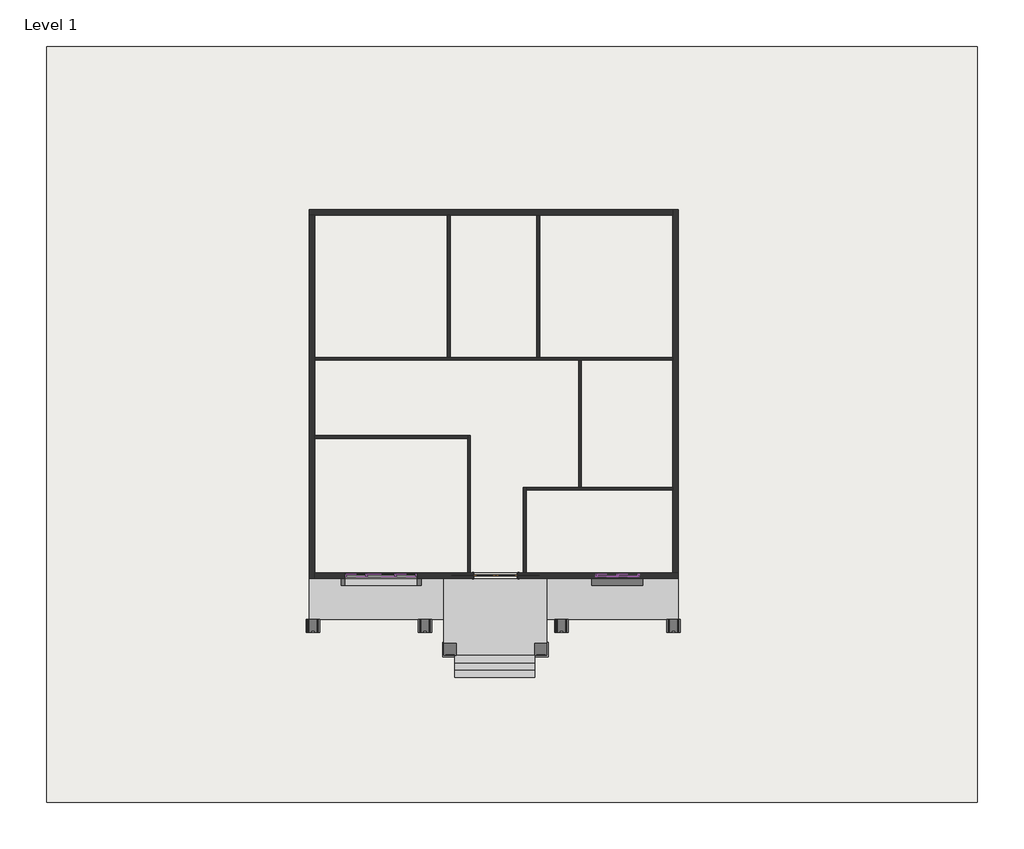
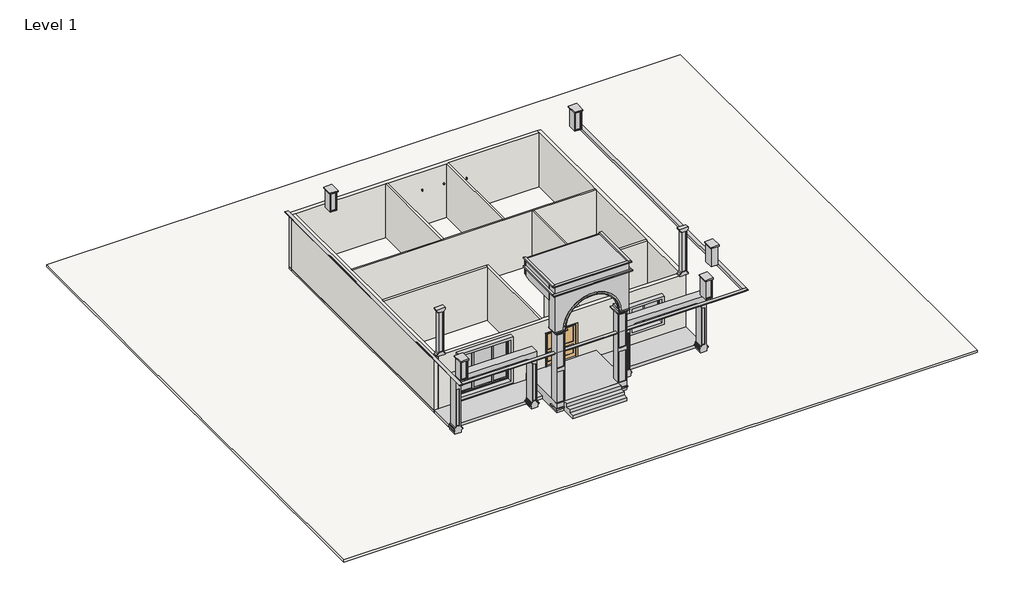
# One storey: 17 members, 12 walls, 5 plates, 2 slabs, 1 door, 1 proxy.
"""IFC4 building model written with IfcOpenShell, lengths in millimetres."""

from ifc_helpers import new_model, si_unit, frame, origin, origin_with_axes, place, context, project, spatial, polyline, outline, extrude, faceted_brep, transform, mapped, element, save
from components import generic_models_1_generic_models_1_83f40e1e, generic_models_1_generic_models_1_5e55def3, generic_models_1_generic_models_1_a6c1d6b2, door_c75fb906, member_c17f1be2, member_9661c287, member_d7472725, member_6ba65f20, member_82905deb, member_4491d118, system_panel_glazed_f88502f0, system_panel_glazed_214c7444, system_panel_glazed_e3982794

model = new_model("IFC4")

# Units and contexts
model_context = context("Model", 3, world=origin())
ifc_project = project(units=[si_unit("LENGTHUNIT", "METRE", prefix="MILLI")], contexts=[model_context])

# Site, building, storey
site = spatial("IfcSite", under=ifc_project)
building = spatial("IfcBuilding", under=site)
storey = spatial("IfcBuildingStorey", under=building, Name="Level 1", Elevation=0.0)

# Proxy
placement = place(None, origin())
generic_models_1_generic_models_1_shape = generic_models_1_generic_models_1_83f40e1e(model_context)
generic_models_1_generic_models_1_2_shape = generic_models_1_generic_models_1_5e55def3(model_context)
generic_models_1_generic_models_1_3_shape = generic_models_1_generic_models_1_a6c1d6b2(model_context)
element("IfcBuildingElementProxy", 1, Name="Generic Models 1 : Generic Models 1", ObjectType="Generic Models 1 : Generic Models 1", at=placement, inside=storey, context=model_context, shape_type="MappedRepresentation", body=[
    mapped(generic_models_1_generic_models_1_shape, transform((0.0, 0.0, 0.0), x_axis=(1.0, 0.0, 0.0), y_axis=(0.0, 1.0, 0.0), z_axis=(0.0, 0.0, 1.0))),
    mapped(generic_models_1_generic_models_1_2_shape, transform((0.0, 0.0, 0.0), x_axis=(1.0, 0.0, 0.0), y_axis=(0.0, 1.0, 0.0), z_axis=(0.0, 0.0, 1.0))),
    mapped(generic_models_1_generic_models_1_3_shape, transform((0.0, 0.0, 0.0), x_axis=(1.0, 0.0, 0.0), y_axis=(0.0, 1.0, 0.0), z_axis=(0.0, 0.0, 1.0))),
])

# Door
door_shape = door_c75fb906(model_context)
element("IfcDoor", 2, ObjectType="Door-Interior-Double-Pocket-2_Panel-Wood : 72\" x 84\"", at=placement, inside=storey, context=model_context, shape_type="MappedRepresentation", body=[
    mapped(door_shape, transform((-962.0249265, -5957.4949916, 609.6), x_axis=(-1.0, 0.0, 0.0), y_axis=(0.0, -1.0, 0.0), z_axis=(0.0, 0.0, 1.0))),
])

# Members
member_shape = member_c17f1be2(model_context)
element("IfcMember", 3, ObjectType="Rectangular Mullion : 2.5\" x 5\" rectangular", at=placement, inside=storey, context=model_context, shape_type="MappedRepresentation", body=[
    mapped(member_shape, transform((-4302.1249265, -5957.4949916, 3352.8), x_axis=(0.0, 0.0, 1.0), y_axis=(0.0, -1.0, 0.0), z_axis=(1.0, 0.0, 0.0))),
])
element("IfcMember", 4, ObjectType="Rectangular Mullion : 2.5\" x 5\" rectangular", at=placement, inside=storey, context=model_context, shape_type="MappedRepresentation", body=[
    mapped(member_shape, transform((-6403.9749265, -5957.4949916, 3352.8), x_axis=(0.0, 0.0, 1.0), y_axis=(0.0, -1.0, 0.0), z_axis=(1.0, 0.0, 0.0))),
])
element("IfcMember", 5, ObjectType="Rectangular Mullion : 2.5\" x 5\" rectangular", at=placement, inside=storey, context=model_context, shape_type="MappedRepresentation", body=[
    mapped(member_shape, transform((3292.4750735, -5957.4949916, 2743.2), x_axis=(0.0, 0.0, 1.0), y_axis=(0.0, 1.0, 0.0), z_axis=(-1.0, 0.0, 0.0))),
])
element("IfcMember", 6, ObjectType="Rectangular Mullion : 2.5\" x 5\" rectangular", at=placement, inside=storey, context=model_context, shape_type="MappedRepresentation", body=[
    mapped(member_shape, transform((4175.1250735, -5957.4949916, 2743.2), x_axis=(0.0, 0.0, 1.0), y_axis=(0.0, 1.0, 0.0), z_axis=(-1.0, 0.0, 0.0))),
])
element("IfcMember", 7, ObjectType="Rectangular Mullion : 2.5\" x 5\" rectangular", at=placement, inside=storey, context=model_context, shape_type="MappedRepresentation", body=[
    mapped(member_shape, transform((-7223.1249265, -5957.4949916, 685.8), x_axis=(0.0, 0.0, -1.0), y_axis=(0.0, -1.0, 0.0), z_axis=(-1.0, 0.0, 0.0))),
])
element("IfcMember", 8, ObjectType="Rectangular Mullion : 2.5\" x 5\" rectangular", at=placement, inside=storey, context=model_context, shape_type="MappedRepresentation", body=[
    mapped(member_shape, transform((-5121.2749265, -5957.4949916, 685.8), x_axis=(0.0, 0.0, -1.0), y_axis=(0.0, -1.0, 0.0), z_axis=(-1.0, 0.0, 0.0))),
])
element("IfcMember", 9, ObjectType="Rectangular Mullion : 2.5\" x 5\" rectangular", at=placement, inside=storey, context=model_context, shape_type="MappedRepresentation", body=[
    mapped(member_shape, transform((4994.2750735, -5957.4949916, 1219.2), x_axis=(0.0, 0.0, -1.0), y_axis=(0.0, 1.0, 0.0), z_axis=(1.0, 0.0, 0.0))),
])
element("IfcMember", 10, ObjectType="Rectangular Mullion : 2.5\" x 5\" rectangular", at=placement, inside=storey, context=model_context, shape_type="MappedRepresentation", body=[
    mapped(member_shape, transform((4111.6250735, -5957.4949916, 1219.2), x_axis=(0.0, 0.0, -1.0), y_axis=(0.0, 1.0, 0.0), z_axis=(1.0, 0.0, 0.0))),
])
member_2_shape = member_9661c287(model_context)
element("IfcMember", 11, ObjectType="Rectangular Mullion : 2.5\" x 5\" rectangular", at=placement, inside=storey, context=model_context, shape_type="MappedRepresentation", body=[
    mapped(member_2_shape, transform((-6372.2249265, -5957.4949916, 685.8), x_axis=(1.0, 0.0, 0.0), y_axis=(0.0, -1.0, 0.0), z_axis=(0.0, 0.0, -1.0))),
])
element("IfcMember", 12, ObjectType="Rectangular Mullion : 2.5\" x 5\" rectangular", at=placement, inside=storey, context=model_context, shape_type="MappedRepresentation", body=[
    mapped(member_2_shape, transform((-5153.0249265, -5957.4949916, 685.8), x_axis=(1.0, 0.0, 0.0), y_axis=(0.0, -1.0, 0.0), z_axis=(0.0, 0.0, -1.0))),
])
member_3_shape = member_d7472725(model_context)
element("IfcMember", 13, ObjectType="Rectangular Mullion : 2.5\" x 5\" rectangular", at=placement, inside=storey, context=model_context, shape_type="MappedRepresentation", body=[
    mapped(member_3_shape, transform((-6340.4749265, -5957.4949916, 685.8), x_axis=(0.0, 0.0, -1.0), y_axis=(0.0, -1.0, 0.0), z_axis=(-1.0, 0.0, 0.0))),
])
element("IfcMember", 14, ObjectType="Rectangular Mullion : 2.5\" x 5\" rectangular", at=placement, inside=storey, context=model_context, shape_type="MappedRepresentation", body=[
    mapped(member_3_shape, transform((-5184.7749265, -5957.4949916, 3352.8), x_axis=(0.0, 0.0, 1.0), y_axis=(0.0, -1.0, 0.0), z_axis=(1.0, 0.0, 0.0))),
])
member_4_shape = member_6ba65f20(model_context)
element("IfcMember", 15, ObjectType="Rectangular Mullion : 2.5\" x 5\" rectangular", at=placement, inside=storey, context=model_context, shape_type="MappedRepresentation", body=[
    mapped(member_4_shape, transform((-7286.6249265, -5957.4949916, 3352.8), x_axis=(-1.0, 0.0, 0.0), y_axis=(0.0, -1.0, 0.0), z_axis=(0.0, 0.0, 1.0))),
])
element("IfcMember", 16, ObjectType="Rectangular Mullion : 2.5\" x 5\" rectangular", at=placement, inside=storey, context=model_context, shape_type="MappedRepresentation", body=[
    mapped(member_4_shape, transform((-4238.6249265, -5957.4949916, 685.8), x_axis=(1.0, 0.0, 0.0), y_axis=(0.0, -1.0, 0.0), z_axis=(0.0, 0.0, -1.0))),
])
member_5_shape = member_82905deb(model_context)
element("IfcMember", 17, ObjectType="Rectangular Mullion : 2.5\" x 5\" rectangular", at=placement, inside=storey, context=model_context, shape_type="MappedRepresentation", body=[
    mapped(member_5_shape, transform((4143.3750735, -5957.4949916, 1219.2), x_axis=(-1.0, 0.0, 0.0), y_axis=(0.0, 1.0, 0.0), z_axis=(0.0, 0.0, -1.0))),
])
member_6_shape = member_4491d118(model_context)
element("IfcMember", 18, ObjectType="Rectangular Mullion : 2.5\" x 5\" rectangular", at=placement, inside=storey, context=model_context, shape_type="MappedRepresentation", body=[
    mapped(member_6_shape, transform((5057.7750735, -5957.4949916, 2743.2), x_axis=(1.0, 0.0, 0.0), y_axis=(0.0, 1.0, 0.0), z_axis=(0.0, 0.0, 1.0))),
])
element("IfcMember", 19, ObjectType="Rectangular Mullion : 2.5\" x 5\" rectangular", at=placement, inside=storey, context=model_context, shape_type="MappedRepresentation", body=[
    mapped(member_6_shape, transform((3228.9750735, -5957.4949916, 1219.2), x_axis=(-1.0, 0.0, 0.0), y_axis=(0.0, 1.0, 0.0), z_axis=(0.0, 0.0, -1.0))),
])

# Plates
system_panel_glazed_shape = system_panel_glazed_f88502f0(model_context)
element("IfcPlate", 20, ObjectType="System Panel : Glazed", at=placement, inside=storey, context=model_context, shape_type="MappedRepresentation", body=[
    mapped(system_panel_glazed_shape, transform((-6813.5499265, -5957.4949916, 749.3), x_axis=(1.0, 0.0, 0.0), y_axis=(0.0, 1.0, 0.0), z_axis=(0.0, 0.0, 1.0))),
])
element("IfcPlate", 21, ObjectType="System Panel : Glazed", at=placement, inside=storey, context=model_context, shape_type="MappedRepresentation", body=[
    mapped(system_panel_glazed_shape, transform((-4711.6999265, -5957.4949916, 749.3), x_axis=(1.0, 0.0, 0.0), y_axis=(0.0, 1.0, 0.0), z_axis=(0.0, 0.0, 1.0))),
])
system_panel_glazed_2_shape = system_panel_glazed_214c7444(model_context)
element("IfcPlate", 22, ObjectType="System Panel : Glazed", at=placement, inside=storey, context=model_context, shape_type="MappedRepresentation", body=[
    mapped(system_panel_glazed_2_shape, transform((-5762.6249265, -5957.4949916, 749.3), x_axis=(1.0, 0.0, 0.0), y_axis=(0.0, 1.0, 0.0), z_axis=(0.0, 0.0, 1.0))),
])
system_panel_glazed_3_shape = system_panel_glazed_e3982794(model_context)
element("IfcPlate", 23, ObjectType="System Panel : Glazed", at=placement, inside=storey, context=model_context, shape_type="MappedRepresentation", body=[
    mapped(system_panel_glazed_3_shape, transform((4584.7000735, -5957.4949916, 1282.7), x_axis=(-1.0, 0.0, 0.0), y_axis=(0.0, -1.0, 0.0), z_axis=(0.0, 0.0, 1.0))),
])
element("IfcPlate", 24, ObjectType="System Panel : Glazed", at=placement, inside=storey, context=model_context, shape_type="MappedRepresentation", body=[
    mapped(system_panel_glazed_3_shape, transform((3702.0500735, -5957.4949916, 1282.7), x_axis=(-1.0, 0.0, 0.0), y_axis=(0.0, -1.0, 0.0), z_axis=(0.0, 0.0, 1.0))),
])

# Slabs
element("IfcSlab", 25, ObjectType="6\" floor", at=placement, inside=storey, context=model_context, shape_type="SweptSolid", body=[
    extrude(outline(polyline([(6696.0750735, 9396.8050084), (6696.0750735, -6071.7949916), (-8772.5249265, -6071.7949916), (-8772.5249265, 9396.8050084), (6696.0750735, 9396.8050084)])), origin_with_axes(), (0.0, 0.0, 1.0), 152.4),
])
element("IfcSlab", 26, ObjectType="6\" floor", at=placement, inside=storey, context=model_context, shape_type="SweptSolid", body=[
    extrude(outline(polyline([(19231.1554065, 16228.5987649), (19231.1554065, -15470.6012351), (-19783.2445935, -15470.6012351), (-19783.2445935, 16228.5987649), (19231.1554065, 16228.5987649)])), frame((0.0, 0.0, -152.4), z_axis=(0.0, 0.0, 1.0), x_axis=(1.0, 0.0, 0.0)), (0.0, 0.0, 1.0), 152.4),
])

# Walls
element("IfcWall", 27, ObjectType="4.5\" wall", at=placement, inside=storey, context=model_context, shape_type="SweptSolid", body=[
    extrude(outline(polyline([(-2981.3249265, 3186.5050084), (-2981.3249265, 9168.2050084), (-2867.0249265, 9168.2050084), (-2867.0249265, 3186.5050084), (-2981.3249265, 3186.5050084)])), origin_with_axes(), (0.0, 0.0, 1.0), 3657.6),
])
element("IfcWall", 28, ObjectType="4.5\" wall", at=placement, inside=storey, context=model_context, shape_type="Brep", body=[
    faceted_brep([(6467.4750735, 3186.5050084, 0.0), (885.8250735, 3186.5050084, 0.0), (771.5250735, 3186.5050084, 0.0), (-2867.0249265, 3186.5050084, 0.0), (-2981.3249265, 3186.5050084, 0.0), (-8543.9249265, 3186.5050084, 0.0), (-8543.9249265, 3186.5050084, 3657.6), (-2981.3249265, 3186.5050084, 3657.6), (-2867.0249265, 3186.5050084, 3657.6), (771.5250735, 3186.5050084, 3657.6), (885.8250735, 3186.5050084, 3657.6), (6467.4750735, 3186.5050084, 3657.6), (6467.4750735, 3072.2050084, 0.0), (6467.4750735, 3072.2050084, 3657.6), (2632.0750735, 3072.2050084, 3657.6), (2517.7750735, 3072.2050084, 3657.6), (-8543.9249265, 3072.2050084, 3657.6), (-8543.9249265, 3072.2050084, 0.0), (2517.7750735, 3072.2050084, 0.0), (2632.0750735, 3072.2050084, 0.0)], [[[0, 1, 2, 3, 4, 5, 6, 7, 8, 9, 10, 11]], [[12, 13, 14, 15, 16, 17, 18, 19]], [[5, 4, 3, 2, 1, 0, 12, 19, 18, 17]], [[6, 5, 17, 16]], [[0, 11, 13, 12]], [[11, 10, 9, 8, 7, 6, 16, 15, 14, 13]]]),
])
element("IfcWall", 29, ObjectType="4.5\" wall", at=placement, inside=storey, context=model_context, shape_type="SweptSolid", body=[
    extrude(outline(polyline([(771.5250735, 3186.5050084), (771.5250735, 9168.2050084), (885.8250735, 9168.2050084), (885.8250735, 3186.5050084), (771.5250735, 3186.5050084)])), origin_with_axes(), (0.0, 0.0, 1.0), 3657.6),
])
element("IfcWall", 30, ObjectType="4.5\" wall", at=placement, inside=storey, context=model_context, shape_type="SweptSolid", body=[
    extrude(outline(polyline([(2517.7750735, -2261.7949916), (2517.7750735, 3072.2050084), (2632.0750735, 3072.2050084), (2632.0750735, -2261.7949916), (2517.7750735, -2261.7949916)])), origin_with_axes(), (0.0, 0.0, 1.0), 3657.6),
])
element("IfcWall", 31, ObjectType="4.5\" wall", at=placement, inside=storey, context=model_context, shape_type="Brep", body=[
    faceted_brep([(314.3250735, -2376.0949916, 0.0), (6467.4750735, -2376.0949916, 0.0), (6467.4750735, -2376.0949916, 3657.6), (314.3250735, -2376.0949916, 3657.6), (314.3250735, -2261.7949916, 0.0), (314.3250735, -2261.7949916, 3657.6), (2517.7750735, -2261.7949916, 3657.6), (2632.0750735, -2261.7949916, 3657.6), (6467.4750735, -2261.7949916, 3657.6), (6467.4750735, -2261.7949916, 0.0), (2632.0750735, -2261.7949916, 0.0), (2517.7750735, -2261.7949916, 0.0)], [[[0, 1, 2, 3]], [[4, 5, 6, 7, 8, 9, 10, 11]], [[1, 0, 4, 11, 10, 9]], [[2, 1, 9, 8]], [[0, 3, 5, 4]], [[3, 2, 8, 7, 6, 5]]]),
])
element("IfcWall", 32, ObjectType="4.5\" wall", at=placement, inside=storey, context=model_context, shape_type="Brep", body=[
    faceted_brep([(314.3250735, -5843.1949916, 0.0), (314.3250735, -2376.0949916, 0.0), (314.3250735, -2261.7949916, 0.0), (314.3250735, -2261.7949916, 3657.6), (314.3250735, -2376.0949916, 3657.6), (314.3250735, -5843.1949916, 3657.6), (200.0250735, -5843.1949916, 0.0), (200.0250735, -5843.1949916, 3657.6), (200.0250735, -2261.7949916, 3657.6), (200.0250735, -2261.7949916, 0.0)], [[[0, 1, 2, 3, 4, 5]], [[6, 7, 8, 9]], [[2, 1, 0, 6, 9]], [[0, 5, 7, 6]], [[3, 2, 9, 8]], [[5, 4, 3, 8, 7]]]),
])
element("IfcWall", 33, ObjectType="4.5\" wall", at=placement, inside=storey, context=model_context, shape_type="Brep", body=[
    faceted_brep([(-2022.4749265, -5843.1949916, 0.0), (-2022.4749265, -90.0949916, 0.0), (-2022.4749265, -90.0949916, 3657.6), (-2022.4749265, -5843.1949916, 3657.6), (-2136.7749265, -5843.1949916, 0.0), (-2136.7749265, -5843.1949916, 3657.6), (-2136.7749265, -204.3949916, 3657.6), (-2136.7749265, -90.0949916, 3657.6), (-2136.7749265, -90.0949916, 0.0), (-2136.7749265, -204.3949916, 0.0)], [[[0, 1, 2, 3]], [[4, 5, 6, 7, 8, 9]], [[1, 0, 4, 9, 8]], [[0, 3, 5, 4]], [[2, 1, 8, 7]], [[3, 2, 7, 6, 5]]]),
])
element("IfcWall", 34, ObjectType="4.5\" wall", at=placement, inside=storey, context=model_context, shape_type="SweptSolid", body=[
    extrude(outline(polyline([(-8543.9249265, -90.0949916), (-2136.7749265, -90.0949916), (-2136.7749265, -204.3949916), (-8543.9249265, -204.3949916), (-8543.9249265, -90.0949916)])), origin_with_axes(), (0.0, 0.0, 1.0), 3657.6),
])
element("IfcWall", 35, ObjectType="9\" wall", at=placement, inside=storey, context=model_context, shape_type="Brep", body=[
    faceted_brep([(-8772.5249265, 9168.2050084, 0.0), (-8543.9249265, 9168.2050084, 0.0), (-2981.3249265, 9168.2050084, 0.0), (-2867.0249265, 9168.2050084, 0.0), (771.5250735, 9168.2050084, 0.0), (885.8250735, 9168.2050084, 0.0), (6467.4750735, 9168.2050084, 0.0), (6467.4750735, 9168.2050084, 3657.6), (885.8250735, 9168.2050084, 3657.6), (771.5250735, 9168.2050084, 3657.6), (-2867.0249265, 9168.2050084, 3657.6), (-2981.3249265, 9168.2050084, 3657.6), (-8543.9249265, 9168.2050084, 3657.6), (-8772.5249265, 9168.2050084, 3657.6), (-8772.5249265, 9396.8050084, 0.0), (-8772.5249265, 9396.8050084, 3657.6), (6467.4750735, 9396.8050084, 3657.6), (6467.4750735, 9396.8050084, 0.0)], [[[0, 1, 2, 3, 4, 5, 6, 7, 8, 9, 10, 11, 12, 13]], [[14, 15, 16, 17]], [[6, 5, 4, 3, 2, 1, 0, 14, 17]], [[0, 13, 15, 14]], [[7, 6, 17, 16]], [[13, 12, 11, 10, 9, 8, 7, 16, 15]]]),
])
element("IfcWall", 36, ObjectType="9\" wall", at=placement, inside=storey, context=model_context, shape_type="Brep", body=[
    faceted_brep([(-8543.9249265, -6071.7949916, 0.0), (-8543.9249265, -5843.1949916, 0.0), (-8543.9249265, -204.3949916, 0.0), (-8543.9249265, -90.0949916, 0.0), (-8543.9249265, 3072.2050084, 0.0), (-8543.9249265, 3186.5050084, 0.0), (-8543.9249265, 9168.2050084, 0.0), (-8543.9249265, 9168.2050084, 3657.6), (-8543.9249265, 3186.5050084, 3657.6), (-8543.9249265, 3072.2050084, 3657.6), (-8543.9249265, -90.0949916, 3657.6), (-8543.9249265, -204.3949916, 3657.6), (-8543.9249265, -5843.1949916, 3657.6), (-8543.9249265, -6071.7949916, 3657.6), (-8772.5249265, -6071.7949916, 0.0), (-8772.5249265, -6071.7949916, 3657.6), (-8772.5249265, 9168.2050084, 3657.6), (-8772.5249265, 9168.2050084, 0.0)], [[[0, 1, 2, 3, 4, 5, 6, 7, 8, 9, 10, 11, 12, 13]], [[14, 15, 16, 17]], [[6, 5, 4, 3, 2, 1, 0, 14, 17]], [[0, 13, 15, 14]], [[7, 6, 17, 16]], [[13, 12, 11, 10, 9, 8, 7, 16, 15]]]),
])
element("IfcWall", 37, ObjectType="9\" wall", at=placement, inside=storey, context=model_context, shape_type="Brep", body=[
    faceted_brep([(6696.0750735, -5843.1949916, 0.0), (6467.4750735, -5843.1949916, 0.0), (314.3250735, -5843.1949916, 0.0), (200.0250735, -5843.1949916, 0.0), (-2022.4749265, -5843.1949916, 0.0), (-2136.7749265, -5843.1949916, 0.0), (-8543.9249265, -5843.1949916, 0.0), (-8543.9249265, -5843.1949916, 3657.6), (-2136.7749265, -5843.1949916, 3657.6), (-2022.4749265, -5843.1949916, 3657.6), (200.0250735, -5843.1949916, 3657.6), (314.3250735, -5843.1949916, 3657.6), (6467.4750735, -5843.1949916, 3657.6), (6696.0750735, -5843.1949916, 3657.6), (-22.2249265, -5843.1949916, 2768.6), (-1901.8249265, -5843.1949916, 2768.6), (-1901.8249265, -5843.1949916, 609.6), (-22.2249265, -5843.1949916, 609.6), (5057.7750735, -5843.1949916, 1219.2), (5057.7750735, -5843.1949916, 2743.2), (3228.9750735, -5843.1949916, 2743.2), (3228.9750735, -5843.1949916, 1219.2), (-7286.6249265, -5843.1949916, 3352.8), (-7286.6249265, -5843.1949916, 685.8), (-4238.6249265, -5843.1949916, 685.8), (-4238.6249265, -5843.1949916, 3352.8), (-8543.9249265, -6071.7949916, 0.0), (6696.0750735, -6071.7949916, 0.0), (6696.0750735, -6071.7949916, 3657.6), (-8543.9249265, -6071.7949916, 3657.6), (-1901.8249265, -6071.7949916, 2768.6), (-22.2249265, -6071.7949916, 2768.6), (-22.2249265, -6071.7949916, 609.6), (-1901.8249265, -6071.7949916, 609.6), (5057.7750735, -6071.7949916, 2743.2), (5057.7750735, -6071.7949916, 1219.2), (3228.9750735, -6071.7949916, 1219.2), (3228.9750735, -6071.7949916, 2743.2), (-7286.6249265, -6071.7949916, 685.8), (-7286.6249265, -6071.7949916, 3352.8), (-4238.6249265, -6071.7949916, 3352.8), (-4238.6249265, -6071.7949916, 685.8), (-2816.2249265, -5978.1324916, 2768.6), (-2816.2249265, -5936.8574916, 2768.6), (-1901.8249265, -5936.8574916, 2768.6), (-22.2249265, -5936.8574916, 2768.6), (892.1750735, -5936.8574916, 2768.6), (892.1750735, -5978.1324916, 2768.6), (-22.2249265, -5978.1324916, 2768.6), (-1901.8249265, -5978.1324916, 2768.6), (-2816.2249265, -5978.1324916, 609.6), (-1901.8249265, -5978.1324916, 609.6), (-22.2249265, -5978.1324916, 609.6), (892.1750735, -5978.1324916, 609.6), (892.1750735, -5936.8574916, 609.6), (-22.2249265, -5936.8574916, 609.6), (-1901.8249265, -5936.8574916, 609.6), (-2816.2249265, -5936.8574916, 609.6)], [[[0, 1, 2, 3, 4, 5, 6, 7, 8, 9, 10, 11, 12, 13], [14, 15, 16, 17], [18, 19, 20, 21], [22, 23, 24, 25]], [[26, 27, 28, 29], [30, 31, 32, 33], [34, 35, 36, 37], [38, 39, 40, 41]], [[6, 5, 4, 3, 2, 1, 0, 27, 26]], [[0, 13, 28, 27]], [[7, 6, 26, 29]], [[42, 43, 44, 15, 14, 45, 46, 47, 48, 31, 30, 49]], [[50, 51, 33, 32, 52, 53, 54, 55, 17, 16, 56, 57]], [[42, 49, 51, 50]], [[49, 30, 33, 51]], [[31, 48, 52, 32]], [[48, 47, 53, 52]], [[47, 46, 54, 53]], [[46, 45, 55, 54]], [[45, 14, 17, 55]], [[15, 44, 56, 16]], [[44, 43, 57, 56]], [[43, 42, 50, 57]], [[18, 35, 34, 19]], [[19, 34, 37, 20]], [[20, 37, 36, 21]], [[35, 18, 21, 36]], [[38, 23, 22, 39]], [[39, 22, 25, 40]], [[24, 41, 40, 25]], [[23, 38, 41, 24]], [[13, 12, 11, 10, 9, 8, 7, 29, 28]]]),
])
element("IfcWall", 38, ObjectType="9\" wall", at=placement, inside=storey, context=model_context, shape_type="Brep", body=[
    faceted_brep([(6467.4750735, 9396.8050084, 0.0), (6467.4750735, 9168.2050084, 0.0), (6467.4750735, 3186.5050084, 0.0), (6467.4750735, 3072.2050084, 0.0), (6467.4750735, -2261.7949916, 0.0), (6467.4750735, -2376.0949916, 0.0), (6467.4750735, -5843.1949916, 0.0), (6467.4750735, -5843.1949916, 3657.6), (6467.4750735, -2376.0949916, 3657.6), (6467.4750735, -2261.7949916, 3657.6), (6467.4750735, 3072.2050084, 3657.6), (6467.4750735, 3186.5050084, 3657.6), (6467.4750735, 9168.2050084, 3657.6), (6467.4750735, 9396.8050084, 3657.6), (6696.0750735, 9396.8050084, 0.0), (6696.0750735, 9396.8050084, 3657.6), (6696.0750735, -5843.1949916, 3657.6), (6696.0750735, -5843.1949916, 0.0)], [[[0, 1, 2, 3, 4, 5, 6, 7, 8, 9, 10, 11, 12, 13]], [[14, 15, 16, 17]], [[6, 5, 4, 3, 2, 1, 0, 14, 17]], [[0, 13, 15, 14]], [[7, 6, 17, 16]], [[13, 12, 11, 10, 9, 8, 7, 16, 15]]]),
])

save(model, "model.ifc")

# Revit data of these elements
# Type "Door-Interior-Double-Pocket-2_Panel-Wood : 72\" x 84\""
#   Type Mark = "8"
#   Assembly Code = "C1020300"
#   Analytic Construction = "Wooden"
#   Top Rail = 0' - 4 11/16"
#   Thickness = 0' - 1 3/8"
#   Thermal Resistance (R) = 2.5876 (h·ft²·°F)/BTU
#   Stiles = 0' - 4 3/4"
#   Rough Width = 12' - 2"
#   Rough Height = 7' - 4 1/2"
#   Panel Width = 3' - 0"
#   Lock Rail = 0' - 7 1/2"
#   Location [instance default] = 3' - 1"
#   Height = 7' - 0"
#   Width = 6' - 0"
#   Heat Transfer Coefficient (U) = 0.3865 BTU/(h·ft²·°F)
#   Bottom Rail = 0' - 9 1/8"
#   Panel Open [instance default] = no
#   Trim Material = Cherry
#   Panel Material = door wood colour
#   Frame Material = door wood colour
#   Visual Light Transmittance = 0
#   Solar Heat Gain Coefficient = 0
#   Wall Closure = (empty or 0)
#   Function = (empty or 0)
# Type "Rectangular Mullion : 2.5\" x 5\" rectangular"
#   built-in parameter 1007304 = 0.416667 (stored number, unit not read)
#   built-in parameter 1007301 = 0.104167 (stored number, unit not read)
#   built-in parameter 1007300 = 0.104167 (stored number, unit not read)
# Type "System Panel : Glazed"
#   Construction Type Id = "GSP4R"
#   Analytic Construction = "1/8 in Pilkington single glazing"
#   Visual Light Transmittance = 0.9
#   Solar Heat Gain Coefficient = 0.86
#   Heat Transfer Coefficient (U) = 1.18115 BTU/(h·ft²·°F)
#   Define Thermal Properties by = 1
# Type "6\" floor"
#   Assembly Code = "B1010"
#   Function = 0
#   Layers, outside or top first: 0' - 6" no material (function 1)
# Type "4.5\" wall"
#   Assembly Code = "B2010"
#   Layers, outside or top first: 0' - 4 1/2" no material (function 1)
# Type "9\" wall"
#   Assembly Code = "B2010"
#   Layers, outside or top first: 0' - 9" "Laminate, Ivory, Matte" (function 1)
# Element 1 (IfcBuildingElementProxy, "Generic Models 1 : Generic Models 1")
#   Phase Created = New Construction
#   Materials on its faces: "Laminate, Ivory, Matte", "Earth"
# Element 2 (IfcDoor, "Door-Interior-Double-Pocket-2_Panel-Wood : 72\" x 84\"")
#   Location = 3' - 1"
#   Panel Open = no
#   Phase Created = New Construction
#   Materials on its faces: "door wood colour", "Cherry"
# Elements 3, 4, 5, 6, 7, 8, 9, 10, 11, 12, 13, 14, 15, 16, 17, 18, 19 (IfcMember, "Rectangular Mullion : 2.5\" x 5\" rectangular")
#   Phase Created = New Construction
# Elements 20, 21, 22, 23, 24 (IfcPlate, "System Panel : Glazed")
#   Phase Created = New Construction
#   Materials on its faces: "Glass"
# Element 25 (IfcSlab, "6\" floor")
#   Height Offset From Level = 0' - 6"
#   Phase Created = New Construction
#   Materials on its faces: "Default Floor"
# Element 26 (IfcSlab, "6\" floor")
#   Height Offset From Level = 0' - 0"
#   Phase Created = New Construction
#   Materials on its faces: "Default Floor"
# Elements 27, 28, 29, 30, 31, 32, 33, 34 (IfcWall, "4.5\" wall")
#   Top Offset = 0' - 0"
#   Base Offset = 0' - 0"
#   wall height = 12' - 0"
#   Phase Created = New Construction
#   Base Constraint = Level 1
#   Top Constraint = Level 2
#   Materials on its faces: "Default Wall"
# Elements 35, 36, 37, 38 (IfcWall, "9\" wall")
#   Top Offset = 0' - 0"
#   Base Offset = 0' - 0"
#   wall height = 12' - 0"
#   Phase Created = New Construction
#   Base Constraint = Level 1
#   Top Constraint = Level 2
#   Materials on its faces: "Laminate, Ivory, Matte"
# Materials
#   "Cherry": class "Wood", colour RGB 226 177 128, transparency 0, Description = "Prunus Serotina", Cost = 0
#   "door wood colour": class "Generic", colour RGB 120 120 120, transparency 0, Cost = 0
#   "Laminate, Ivory, Matte": class "Plastic", colour RGB 247 247 239, transparency 0, Description = "Plastic Laminate - Ivory, Matte", Cost = 0
#   "Earth": class "Generic", colour RGB 97 75 62, transparency 0, Description = "Soil", Cost = 0
#   "Glass": class "Glass", colour RGB 0 128 192, transparency 0.75, Description = "Soda Lime Glass", Cost = 0
#   "Default Floor": colour RGB 128 128 128, transparency 0, Cost = 0
#   "Default Wall": colour RGB 128 128 128, transparency 0, Cost = 0
